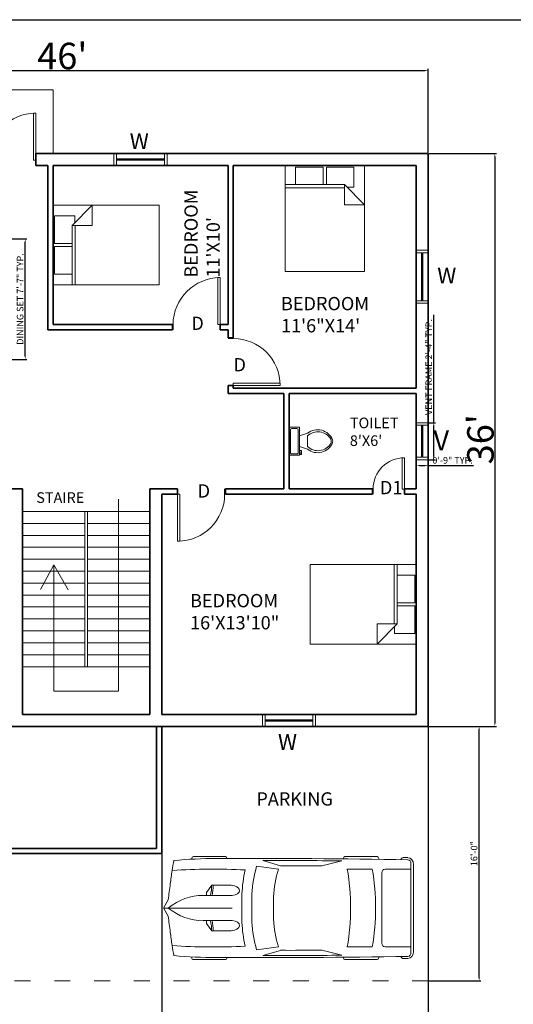
# Model space of a CAD drawing. Units: inches. Extents: x 1662 to 23131, y 1265 to 19127.
# Tile 25 of 26: x 22232 to 22604, y 18361 to 19104. Entities that reach past the tile are written whole.
import ezdxf

# ---------------------------------------------------------------- set-up
doc = ezdxf.new("R2010")
doc.units = ezdxf.units.IN
doc.linetypes.add('ACAD_ISO03W100', pattern=[30, 12, -18])
for name, color, linetype, lineweight in [('A-ANNO-DIMS', 4, 'Continuous', 18), ('A-ANNO-IDEN', 7, 'Continuous', 18), ('A-ANNO-TTLB', 7, 'Continuous', 25), ('A-AREA-IDEN', 7, 'Continuous', 18), ('A-DOOR', 3, 'Continuous', 18), ('A-FLOR-FIXT', 9, 'Continuous', 18), ('A-FLOR-STRS', 7, 'Continuous', 18), ('A-FURN', 8, 'Continuous', 18), ('A-GLAZ', 4, 'Continuous', 18), ('A-SITE-PRKG', 8, 'ACAD_ISO03W100', 18), ('A-SITE-VEHC', 8, 'Continuous', 18), ('A-WALL', 7, 'Continuous', 35)]:
    doc.layers.add(name, color=color, linetype=linetype, lineweight=lineweight)
doc.styles.get("Standard").update_dxf_attribs({"font": 'arial.ttf'})
doc.dimstyles.new('ISO-25', dxfattribs={"dimtxt": 5, "dimasz": 2.5, "dimexe": 1.25, "dimexo": 0.625, "dimtad": 1, "dimlunit": 3, "dimtxsty": 'Standard', "dimcen": 2.5, "dimadec": 0, "dimazin": 0, "dimtfac": 1, "dimtmove": 0, "dimatfit": 3, "dimfxl": 1, "dimarcsym": 0})

# ---------------------------------------------------------------- blocks, each defined once
blk = doc.blocks.new('*U117')
for p, q in [((0, 0), (0, 100)), ((900, 0), (900, 100))]:
    blk.add_line(p, q)
blk.add_lwpolyline([(0, 0), (0, -900), (43.75, -900), (43.75, 0)], close=True)
blk.add_arc((0, 0), 900, 270, 0)
blk = doc.blocks.new('*U121')
for p, q in [((0, 0), (0, -100)), ((-900, 0), (-900, -100))]:
    blk.add_line(p, q)
blk.add_lwpolyline([(0, 0), (0, 900), (-43.75, 900), (-43.75, 0)], close=True)
blk.add_arc((0, 0), 900, 90, 180)
blk = doc.blocks.new('*U120')
for p, q in [((0, 0), (0, -100)), ((-900, 0), (-900, -100))]:
    blk.add_line(p, q)
blk.add_lwpolyline([(0, 0), (0, 900), (-43.75, 900), (-43.75, 0)], close=True)
blk.add_arc((0, 0), 900, 90, 180)
blk = doc.blocks.new('*U118')
for p, q in [((-600, 0), (-600, -100)), ((0, 0), (0, -100))]:
    blk.add_line(p, q)
blk.add_lwpolyline([(0, 0), (0, 600), (-43.75, 600), (-43.75, 0)], close=True)
blk.add_arc((0, 0), 600, 90, 180)
blk = doc.blocks.new('Bed - Queen')
for p, q in [((0, -80.00003), (0, 0)), ((0, 0), (59.99999, 0)), ((59.99999, 0), (59.99999, -80.00003)), ((7.99999, -1.2), (28.79998, -1.2)), ((7.99999, -14.4), (7.99999, -1.2)), ((28.79998, -1.2), (28.79998, -14.4)), ((31.19999, -1.2), (51.99999, -1.2)), ((31.19999, -14.4), (31.19999, -1.2)), ((51.99999, -1.2), (51.99999, -16.4)), ((0, -14.4), (44.8, -14.4)), ((59.99999, -29.6), (44.8, -14.4)), ((44.8, -14.4), (44.8, -29.6)), ((44.8, -16.8), (0, -16.8)), ((51.99999, -16.4), (46.79936, -16.4)), ((44.8, -29.6), (59.99999, -29.6)), ((59.99999, -80.00003), (0, -80.00003))]:
    blk.add_line(p, q)
blk = doc.blocks.new('Toilet - top')
for p, q in [((9.5, -6), (9.5, -2)), ((-10, -8.5), (-8, -8.5)), ((-10, -9.5), (-10, -8.5)), ((-7, -9.5), (-10, -9.5)), ((-8, -8.5), (-8, -8)), ((-7, -8), (-7, -9.5)), ((-4, -8), (-6, -14)), ((4, -14), (-4, -14)), ((4, -8), (6, -14))]:
    blk.add_line(p, q)
blk.add_lwpolyline([(10.5, -8), (10.5, 0), (-10.5, 0), (-10.5, -8)], close=True)
for points in [[(-9.5, -2), (-9.5, -6)], [(8.5, -1), (-8.5, -1)], [(-8.5, -7), (8.5, -7)]]:
    blk.add_lwpolyline(points)
for centre, radius, start, end in [((-8.62, -1.88), 0.884, 81.8699, 188.1301), ((-8.62, -6.12), 0.884, 171.8699, 278.1301), ((8.62, -1.88), 0.884, 351.8699, 98.1301), ((8.62, -6.12), 0.884, 261.8699, 8.1301), ((3.52, -21.58), 12.17, 141.46911, 247.97143), ((4.2, -21.82), 11.33, 136.36773, 238.94682), ((-3.52, -21.58), 12.17, 292.02843, 38.53071), ((-4.2, -21.82), 11.33, 301.05301, 43.63209), ((0, -27.88), 4, 245.73182, 294.26817), ((0, -29), 4, 254.86053, 285.13947)]:
    blk.add_arc(centre, radius, start, end)
blk = doc.blocks.new('*U66')
for p, q in [((536, 950), (536, 936)), ((1182, 988), (568, 988)), ((1214, 950), (1214, 950)), ((3440, 942), (3440, 950)), ((3472, 988), (4087, 988)), ((4119, 950), (4119, 934)), ((1779, 801), (2195, 746)), ((2235, 810), (1899, 912)), ((3412, 904), (3030, 807)), ((4736, -851), (4736, 851)), ((4785, -832), (4785, 832)), ((3516, 746), (3994, 746)), ((4179, 670), (4179, -670)), ((4736, 746), (4242, 746)), ((820, 295), (918, 436)), ((918, 436), (1294, 436)), ((756, 241), (1313, 241)), ((816, 241), (816, 283)), ((1496, -274), (1496, 274)), ((1690, -267), (1690, 267)), ((2102, 216), (2102, -216)), ((4736, -267), (4736, 267)), ((83, 156), (3, 10)), ((0, 0), (1313, 0)), ((3, -10), (83, -156)), ((756, -241), (1313, -241)), ((816, -241), (816, -283)), ((820, -295), (918, -436)), ((918, -436), (1294, -436)), ((2195, -746), (1779, -801)), ((3994, -746), (3516, -746)), ((4242, -746), (4736, -746)), ((536, -950), (536, -936)), ((2235, -810), (1899, -912)), ((3412, -904), (3030, -807)), ((3440, -942), (3440, -950)), ((4119, -950), (4119, -934)), ((1182, -988), (568, -988)), ((1214, -950), (1214, -950)), ((3472, -988), (4087, -988))]:
    blk.add_line(p, q)
for centre, major_axis, ratio, start_param, end_param in [((1046, -12468), (0, 13417), 0.842304, 0.00281, 0.075598), ((568, 950), (0, -37.6), 0.842304, 3.141593, 4.712389), ((1638, -268113), (0, 269063), 0.842304, -0.013397, 0.002797), ((1182, 950), (0, 37.6), 0.842304, -1.570796, 0), ((3472, 950), (0, -37.6), 0.842304, 3.141593, 4.712389), ((4087, 950), (0, 37.6), 0.842304, -1.570796, 0), ((4588, 910), (0, 56.4), 0.842304, -0.013017, 1.249894), ((1638, -268131), (0, 269121), 0.842304, -0.013397, -0.013017), ((4673, 832), (0, -133), 0.842304, 1.570796, 3.128196), ((6757, -699), (0, 7958), 0.842304, 1.367076, 1.39176), ((952, -15087), (0, -15833), 0.842304, 3.096046, 3.200911), ((3436, 137), (0, 2077), 0.842304, 1.245306, 1.50788), ((1638, -268113), (0, -269025), 0.842304, 3.133765, 3.140441), ((2433, -93125), (0, -93935), 0.842304, 3.134049, 3.144098), ((4673, 851), (0, -75.2), 0.842304, 1.570796, 3.128196), ((6583, -699), (0, -7755), 0.842304, 4.528606, 4.561838), ((3414, 137), (0, -2280), 0.842304, 4.449482, 4.652344), ((3800, 71), (0, -2021), 0.842304, 4.372215, 4.640744), ((434, 0), (0, 3734), 0.842304, 4.511394, 4.913384), ((912, 0), (0, 3734), 0.842304, 4.511394, 4.913384), ((4242, 670), (0, 75.2), 0.842304, 0, 1.570796), ((-5194, 1331), (0, -6374), 0.842304, 1.385369, 1.434372), ((331, 432), (0, 696), 0.842304, 4.435146, 4.718221), ((361, 432), (0, 696), 0.842304, 4.435146, 4.718221), ((1290, 339), (161, -9), 0.603834, -1.395552, 1.581315), ((756, -1185), (0, 1427), 0.842304, 0, 0.590319), ((832, 283), (0, 18.8), 0.842304, 0.879714, 1.570796), ((16, 0), (0, -18.8), 0.842304, 4.131459, 5.293319), ((-5194, -1331), (0, 6374), 0.842304, -1.434372, -1.385369), ((756, 1185), (0, 1427), 0.842304, 2.551274, 3.141593), ((832, -283), (0, -18.8), 0.842304, 4.712389, 5.403472), ((331, -432), (0, -696), 0.842304, 1.564964, 1.848039), ((361, -432), (0, -696), 0.842304, 1.564964, 1.848039), ((3414, -137), (0, -2280), 0.842304, -1.510751, -1.307889), ((3436, -137), (0, -2077), 0.842304, -1.50788, -1.245306), ((3800, -71), (0, -2021), 0.842304, -1.499151, -1.230623), ((6583, 699), (0, 7755), 0.842304, 1.721348, 1.754579), ((6757, 699), (0, 7958), 0.842304, 1.749832, 1.774517), ((952, 15087), (0, -15833), 0.842304, -0.059319, 0.045547), ((4242, -670), (0, -75.2), 0.842304, 4.712389, 6.283185), ((1046, 12468), (0, -13417), 0.842304, -0.075598, -0.00281), ((1638, 268113), (0, 269063), 0.842304, 3.138796, 3.15499), ((1638, 268113), (0, -269025), 0.842304, 0.001152, 0.007828), ((2433, 93125), (0, -93935), 0.842304, -0.002505, 0.007544), ((4588, -910), (0, -56.4), 0.842304, -1.249894, 0.013017), ((4673, -851), (0, 75.2), 0.842304, 3.15499, 4.712389), ((4673, -832), (0, -133), 0.842304, 0.013397, 1.570796), ((568, -950), (0, 37.6), 0.842304, 1.570796, 3.141593), ((1182, -950), (0, -37.6), 0.842304, 0, 1.570796), ((3472, -950), (0, -37.6), 0.842304, -1.570796, 0), ((4087, -950), (0, 37.6), 0.842304, 3.141593, 4.712389), ((1638, 268131), (0, 269121), 0.842304, 3.15461, 3.15499)]:
    blk.add_ellipse(centre, major_axis=major_axis, ratio=ratio, start_param=start_param, end_param=end_param)
at = {"extrusion": (0, 0, -1)}
blk.add_ellipse((1290, -339), major_axis=(161, 9), ratio=0.603834, start_param=-1.395552, end_param=1.581315, dxfattribs=at)
blk = doc.blocks.new('*D123')
at = {"layer": 'A-ANNO-DIMS', "color": 0, "lineweight": -2, "transparency": 16777216}
for p, q in [((22540.77, 19002.71), (22591.62, 19002.71)), ((22590.37, 19000.21), (22590.37, 18573.21)), ((22540.77, 18570.71), (22591.62, 18570.71))]:
    blk.add_line(p, q, dxfattribs=at)
at = {"layer": 'A-ANNO-DIMS', "color": 0, "transparency": 16777216}
for points in [[(22589.95, 19000.21), (22590.78, 19000.21), (22590.37, 19002.71)], [(22589.95, 18573.21), (22590.78, 18573.21), (22590.37, 18570.71)]]:
    blk.add_solid(points, dxfattribs=at)
at = {"layer": 'Defpoints', "color": 0, "transparency": 16777216}
for p in [(22540.15, 19002.71), (22540.15, 18570.71), (22590.37, 18570.71)]:
    blk.add_point(p, dxfattribs=at)
at = {"layer": 'A-ANNO-DIMS', "color": 0, "transparency": 16777216, "insert": (22579.52, 18787.23), "char_height": 5, "attachment_point": 5, "rotation": 90}
blk.add_mtext("{\\H4x;36'}", dxfattribs=at)
blk = doc.blocks.new('*D124')
at = {"layer": 'A-ANNO-DIMS', "color": 0, "lineweight": -2, "transparency": 16777216}
for p, q in [((21988.15, 19003.33), (21988.15, 19066.63)), ((21990.65, 19065.38), (22537.65, 19065.38)), ((22540.15, 19003.33), (22540.15, 19066.63))]:
    blk.add_line(p, q, dxfattribs=at)
at = {"layer": 'A-ANNO-DIMS', "color": 0, "transparency": 16777216}
for points in [[(21990.65, 19065.79), (21990.65, 19064.96), (21988.15, 19065.38)], [(22537.65, 19065.79), (22537.65, 19064.96), (22540.15, 19065.38)]]:
    blk.add_solid(points, dxfattribs=at)
at = {"layer": 'Defpoints', "color": 0, "transparency": 16777216}
for p in [(22540.15, 19065.38), (21988.15, 19002.71), (22540.15, 19002.71)]:
    blk.add_point(p, dxfattribs=at)
at = {"layer": 'A-ANNO-DIMS', "color": 0, "transparency": 16777216, "insert": (22264.15, 19076.21), "char_height": 5, "attachment_point": 5}
blk.add_mtext("{\\H4x;46'}", dxfattribs=at)
blk = doc.blocks.new('VENT-24-J9X2')
for p, q in [((9, 28), (0, 28)), ((9, 26), (0, 26)), ((4, 26), (4, 2)), ((4.5, 26), (4.5, 2)), ((5, 26), (5, 2)), ((9, 2), (0, 2)), ((9, 0), (0, 0))]:
    blk.add_line(p, q)
blk = doc.blocks.new('WIN-36-J9X2')
for p, q in [((0, 0), (0, 9)), ((2, 0), (2, 9)), ((38, 0), (38, 9)), ((40, 0), (40, 9)), ((38, 5), (2, 5)), ((38, 4.5), (2, 4.5)), ((38, 4), (2, 4))]:
    blk.add_line(p, q)
blk = doc.blocks.new('*D177')
at = {"layer": 'A-ANNO-DIMS', "color": 0, "lineweight": -2, "transparency": 16777216}
for p, q in [((22223.17, 18938.46), (22237.45, 18938.46)), ((22236.2, 18849.96), (22236.2, 18935.96)), ((22223.17, 18847.46), (22237.45, 18847.46))]:
    blk.add_line(p, q, dxfattribs=at)
at = {"layer": 'A-ANNO-DIMS', "color": 0, "transparency": 16777216}
for points in [[(22235.78, 18935.96), (22236.62, 18935.96), (22236.2, 18938.46)], [(22235.78, 18849.96), (22236.62, 18849.96), (22236.2, 18847.46)]]:
    blk.add_solid(points, dxfattribs=at)
at = {"layer": 'Defpoints', "color": 0, "transparency": 16777216}
for p in [(22222.55, 18938.46), (22236.2, 18938.46), (22222.55, 18847.46)]:
    blk.add_point(p, dxfattribs=at)
at = {"layer": 'A-ANNO-DIMS', "color": 0, "transparency": 16777216, "insert": (22232.99, 18892.96), "char_height": 5, "attachment_point": 5, "rotation": 90}
blk.add_mtext('DINING SET 7\'-7" TYP.', dxfattribs=at)
blk = doc.blocks.new('*D181')
at = {"layer": 'A-ANNO-DIMS', "color": 0, "lineweight": -2, "transparency": 16777216}
for p, q in [((22544.35, 18799.71), (22544.35, 18881.15)), ((22540.77, 18799.71), (22545.6, 18799.71)), ((22544.35, 18774.21), (22544.35, 18797.21)), ((22540.77, 18771.71), (22545.6, 18771.71))]:
    blk.add_line(p, q, dxfattribs=at)
at = {"layer": 'A-ANNO-DIMS', "color": 0, "transparency": 16777216}
for points in [[(22543.93, 18797.21), (22544.77, 18797.21), (22544.35, 18799.71)], [(22543.93, 18774.21), (22544.77, 18774.21), (22544.35, 18771.71)]]:
    blk.add_solid(points, dxfattribs=at)
at = {"layer": 'Defpoints', "color": 0, "transparency": 16777216}
for p in [(22540.15, 18799.71), (22544.35, 18799.71), (22540.15, 18771.71)]:
    blk.add_point(p, dxfattribs=at)
at = {"layer": 'A-ANNO-DIMS', "color": 0, "transparency": 16777216, "insert": (22541.21, 18841.68), "char_height": 5, "attachment_point": 5, "rotation": 90}
blk.add_mtext('VENT FRAME 2\'-4" TYP.', dxfattribs=at)
blk = doc.blocks.new('*D182')
at = {"layer": 'A-ANNO-DIMS', "color": 0, "lineweight": -2, "transparency": 16777216}
for p, q in [((22531.15, 18771.08), (22531.15, 18766.26)), ((22540.15, 18771.08), (22540.15, 18766.26)), ((22533.65, 18767.51), (22537.65, 18767.51)), ((22540.15, 18767.51), (22574.38, 18767.51))]:
    blk.add_line(p, q, dxfattribs=at)
at = {"layer": 'A-ANNO-DIMS', "color": 0, "transparency": 16777216}
for points in [[(22533.65, 18767.93), (22533.65, 18767.09), (22531.15, 18767.51)], [(22537.65, 18767.93), (22537.65, 18767.09), (22540.15, 18767.51)]]:
    blk.add_solid(points, dxfattribs=at)
at = {"layer": 'Defpoints', "color": 0, "transparency": 16777216}
for p in [(22531.15, 18771.71), (22540.15, 18771.71), (22540.15, 18767.51)]:
    blk.add_point(p, dxfattribs=at)
at = {"layer": 'A-ANNO-DIMS', "color": 0, "transparency": 16777216, "insert": (22558.51, 18770.69), "char_height": 5, "attachment_point": 5}
blk.add_mtext('0\'-9" TYP.', dxfattribs=at)
blk = doc.blocks.new('*D255')
at = {"layer": 'A-ANNO-DIMS', "color": 0, "lineweight": -2, "transparency": 16777216}
for p, q in [((22339.15, 18570.08), (22339.15, 18310.24)), ((22540.15, 18570.08), (22540.15, 18310.24)), ((22341.65, 18311.49), (22537.65, 18311.49))]:
    blk.add_line(p, q, dxfattribs=at)
at = {"layer": 'A-ANNO-DIMS', "color": 0, "transparency": 16777216}
for points in [[(22341.65, 18311.91), (22341.65, 18311.08), (22339.15, 18311.49)], [(22537.65, 18311.91), (22537.65, 18311.08), (22540.15, 18311.49)]]:
    blk.add_solid(points, dxfattribs=at)
at = {"layer": 'Defpoints', "color": 0, "transparency": 16777216}
for p in [(22339.15, 18570.71), (22540.15, 18570.71), (22540.15, 18311.49)]:
    blk.add_point(p, dxfattribs=at)
at = {"layer": 'A-ANNO-DIMS', "color": 0, "transparency": 16777216, "insert": (22439.65, 18314.67), "char_height": 5, "attachment_point": 5}
blk.add_mtext('16\'-9"', dxfattribs=at)
blk = doc.blocks.new('*D256')
at = {"layer": 'A-ANNO-DIMS', "color": 0, "lineweight": -2, "transparency": 16777216}
for p, q in [((22540.77, 18570.71), (22579.8, 18570.71)), ((22578.55, 18381.21), (22578.55, 18568.21)), ((22540.77, 18378.71), (22579.8, 18378.71))]:
    blk.add_line(p, q, dxfattribs=at)
at = {"layer": 'A-ANNO-DIMS', "color": 0, "transparency": 16777216}
for points in [[(22578.13, 18568.21), (22578.97, 18568.21), (22578.55, 18570.71)], [(22578.13, 18381.21), (22578.97, 18381.21), (22578.55, 18378.71)]]:
    blk.add_solid(points, dxfattribs=at)
at = {"layer": 'Defpoints', "color": 0, "transparency": 16777216}
for p in [(22540.15, 18570.71), (22578.55, 18570.71), (22540.15, 18378.71)]:
    blk.add_point(p, dxfattribs=at)
at = {"layer": 'A-ANNO-DIMS', "color": 0, "transparency": 16777216, "insert": (22575.37, 18474.71), "char_height": 5, "attachment_point": 5, "rotation": 90}
blk.add_mtext('16\'-0"', dxfattribs=at)

msp = doc.modelspace()

# ---------------------------------------------------------------- linework, layer by layer
at = {"layer": 'A-ANNO-TTLB'}
msp.add_lwpolyline([(21860.989, 19103.605), (23130.86, 19103.605), (23130.86, 17867.351), (21860.989, 17867.351)], close=True, dxfattribs=at)
at = {"layer": 'A-FLOR-STRS'}
for p, q in [((22257.149, 19050.71), (22161.274, 19050.71)), ((22257.149, 19002.71), (22257.149, 19050.71)), ((22306.649, 18742.121), (22306.649, 18597.14)), ((22330.149, 18732.71), (22234.149, 18732.71)), ((22281.149, 18615.71), (22281.149, 18732.71)), ((22283.149, 18615.71), (22283.149, 18732.71)), ((22281.149, 18723.71), (22234.149, 18723.71)), ((22330.149, 18723.71), (22283.149, 18723.71)), ((22281.149, 18714.71), (22234.149, 18714.71)), ((22330.149, 18714.71), (22283.149, 18714.71)), ((22281.149, 18705.71), (22234.149, 18705.71)), ((22330.149, 18705.71), (22283.149, 18705.71)), ((22281.149, 18696.71), (22234.149, 18696.71)), ((22330.149, 18696.71), (22283.149, 18696.71)), ((22257.649, 18692.581), (22247.631, 18673.83)), ((22257.649, 18597.14), (22257.649, 18692.581)), ((22257.649, 18692.581), (22268.486, 18673.708)), ((22281.149, 18687.71), (22234.149, 18687.71)), ((22330.149, 18687.71), (22283.149, 18687.71)), ((22281.149, 18678.71), (22234.149, 18678.71)), ((22330.149, 18678.71), (22283.149, 18678.71)), ((22281.149, 18669.71), (22234.149, 18669.71)), ((22330.149, 18669.71), (22283.149, 18669.71)), ((22281.149, 18660.71), (22234.149, 18660.71)), ((22330.149, 18660.71), (22283.149, 18660.71)), ((22281.149, 18651.71), (22234.149, 18651.71)), ((22330.149, 18651.71), (22283.149, 18651.71)), ((22281.149, 18642.71), (22234.149, 18642.71)), ((22330.149, 18642.71), (22283.149, 18642.71)), ((22281.149, 18633.71), (22234.149, 18633.71)), ((22330.149, 18633.71), (22283.149, 18633.71)), ((22281.149, 18624.71), (22234.149, 18624.71)), ((22330.149, 18624.71), (22283.149, 18624.71)), ((22330.149, 18615.71), (22234.149, 18615.71)), ((22306.649, 18597.14), (22257.649, 18597.14))]:
    msp.add_line(p, q, dxfattribs=at)
at = {"layer": 'A-SITE-PRKG'}
for p, q in [((22540.149, 18570.71), (22540.149, 18378.71)), ((22540.149, 18378.71), (21988.149, 18378.71))]:
    msp.add_line(p, q, dxfattribs=at)
at = {"layer": 'A-WALL'}
for p, q in [((22244.149, 18993.71), (22244.149, 19002.71)), ((22244.149, 19002.71), (22540.149, 19002.71)), ((22540.149, 19002.71), (22540.149, 18570.71)), ((22244.149, 18993.71), (22253.149, 18993.71)), ((22253.149, 18869.71), (22253.149, 18993.71)), ((22257.149, 18873.71), (22257.149, 18993.71)), ((22257.149, 18993.71), (22389.149, 18993.71)), ((22389.149, 18873.71), (22389.149, 18993.71)), ((22393.149, 18863.71), (22393.149, 18993.71)), ((22393.149, 18993.71), (22531.149, 18993.71)), ((22531.149, 18993.71), (22531.149, 18825.71)), ((22253.149, 18869.71), (22347.149, 18869.71)), ((22257.149, 18873.71), (22347.149, 18873.71)), ((22347.149, 18869.71), (22347.149, 18873.71)), ((22383.149, 18869.71), (22383.149, 18873.71)), ((22383.149, 18873.71), (22389.149, 18873.71)), ((22383.149, 18869.71), (22389.149, 18869.71)), ((22389.149, 18863.71), (22389.149, 18869.71)), ((22389.149, 18863.71), (22393.149, 18863.71)), ((22389.149, 18821.71), (22389.149, 18827.71)), ((22389.149, 18827.71), (22393.149, 18827.71)), ((22393.149, 18825.71), (22393.149, 18827.71)), ((22393.149, 18825.71), (22531.149, 18825.71)), ((22389.149, 18821.71), (22431.149, 18821.71)), ((22431.149, 18821.71), (22431.149, 18749.71)), ((22435.149, 18821.71), (22435.149, 18749.71)), ((22435.149, 18821.71), (22531.149, 18821.71)), ((22531.149, 18821.71), (22531.149, 18749.71)), ((22225.149, 18749.71), (22234.149, 18749.71)), ((22234.149, 18579.71), (22234.149, 18749.71)), ((22330.149, 18749.71), (22330.149, 18579.71)), ((22330.149, 18749.71), (22351.149, 18749.71)), ((22351.149, 18749.71), (22351.149, 18745.71)), ((22387.149, 18749.71), (22387.149, 18745.71)), ((22387.149, 18749.71), (22419.149, 18749.71)), ((22419.149, 18749.71), (22431.149, 18749.71)), ((22435.149, 18749.71), (22498.149, 18749.71)), ((22498.149, 18745.71), (22498.149, 18749.71)), ((22522.149, 18745.71), (22522.149, 18749.71)), ((22522.149, 18749.71), (22531.149, 18749.71)), ((22339.149, 18745.71), (22339.149, 18579.71)), ((22339.149, 18745.71), (22351.149, 18745.71)), ((22387.149, 18745.71), (22419.149, 18745.71)), ((22419.149, 18745.71), (22498.149, 18745.71)), ((22522.149, 18745.71), (22531.149, 18745.71)), ((22531.149, 18745.71), (22531.149, 18579.71)), ((22531.149, 18662.71), (22531.149, 18662.71)), ((22330.149, 18579.71), (22234.149, 18579.71)), ((22531.149, 18579.71), (22339.149, 18579.71)), ((22540.149, 18570.71), (22213.149, 18570.71)), ((22335.149, 18570.71), (22335.149, 18478.71)), ((22339.149, 18570.71), (22339.149, 18474.71)), ((22339.149, 18474.71), (22079.649, 18474.71)), ((22335.149, 18478.71), (22083.649, 18478.71))]:
    msp.add_line(p, q, dxfattribs=at)

# ---------------------------------------------------------------- block references
at = {"layer": 'A-DOOR', "xscale": 0.0393700787401575, "yscale": 0.0393700787401575, "zscale": 0.0393700787401575}
for name, p in [('*U121', (22244.149, 18997.647)), ('*U121', (22383.149, 18873.647)), ('*U118', (22522.149, 18749.647)), ('*U117', (22351.149, 18745.773))]:
    msp.add_blockref(name, p, dxfattribs=at)
at = {"layer": 'A-DOOR', "xscale": 0.0393700787401575, "yscale": 0.0393700787401575, "zscale": 0.0393700787401575, "rotation": 270}
msp.add_blockref('*U120', (22393.086, 18827.71), dxfattribs=at)
at = {"layer": 'A-FLOR-FIXT', "rotation": 90}
msp.add_blockref('Toilet - top', (22435.149, 18785.71), dxfattribs=at)
at = {"layer": 'A-FURN'}
msp.add_blockref('Bed - Queen', (22432.149, 18993.71), dxfattribs=at)
for p, rotation in [((22257.149, 18903.71), 89.99999999999999), ((22531.149, 18692.71), 270)]:
    msp.add_blockref('Bed - Queen', p, dxfattribs=dict(at, rotation=rotation))
at = {"layer": 'A-GLAZ'}
for name, p in [('WIN-36-J9X2', (22303.149, 18993.71)), ('VENT-24-J9X2', (22531.149, 18771.71)), ('WIN-36-J9X2', (22415.149, 18570.71))]:
    msp.add_blockref(name, p, dxfattribs=at)
at = {"layer": 'A-GLAZ', "rotation": 90}
msp.add_blockref('WIN-36-J9X2', (22540.149, 18889.709), dxfattribs=at)
at = {"layer": 'A-SITE-VEHC', "xscale": 0.0393700787401575, "yscale": 0.0393700787401575, "zscale": 0.0393700787401575}
msp.add_blockref('*U66', (22340.677, 18433.685), dxfattribs=at)

# ---------------------------------------------------------------- texts
at = {"layer": 'A-ANNO-IDEN', "attachment_point": 1}
for s, width, heights, insert, char_height in [('W', 471.52273, [28.462], (22315.012, 19018.01), 12), ('W', 471.52273, [28.462], (22546.949, 18916.716), 12), ('D', 1142.59551, [0], (22361.493, 18879.666), 10), ('D', 1142.59551, [0], (22393.28, 18848.385), 10), ('V', 1142.59551, [20], (22544.061, 18793.863), 15), ('D', 1142.59551, [0], (22366.243, 18753.244), 10), ('D1', 1142.59551, [20], (22503.712, 18755.755), 10), ('W', 471.52273, [28.462], (22426.818, 18564.969), 12)]:
    msp.add_mtext_dynamic_manual_height_columns(s, width=width, gutter_width=12.5, heights=heights, dxfattribs=dict(at, insert=insert, char_height=char_height))
at = {"layer": 'A-AREA-IDEN', "insert": (22356.264, 18909.08), "char_height": 10, "attachment_point": 1, "rotation": 90}
msp.add_mtext_dynamic_manual_height_columns("BEDROOM\\P11'X10'", width=1142.59551, gutter_width=12.5, heights=[277.772], dxfattribs=at)
at = {"layer": 'A-AREA-IDEN', "attachment_point": 1}
for s, insert, char_height in [('BEDROOM\\P11\'6"X14\'', (22429.103, 18894.49), 10), ("TOILET\\P8'X6'", (22481.026, 18803.516), 8), ('STAIRE', (22244.504, 18747.208), 8), ('BEDROOM\\P16\'X13\'10"', (22360.517, 18670.489), 10), ('PARKING', (22410.538, 18520.968), 10)]:
    msp.add_mtext_dynamic_manual_height_columns(s, width=1142.59551, gutter_width=12.5, heights=[277.772], dxfattribs=dict(at, insert=insert, char_height=char_height))

# ---------------------------------------------------------------- dimensions: what is measured, and where the dimension line sits
at = {"layer": 'A-ANNO-DIMS'}
for base, p1, p2, text, override, picture, middle in [((22540.149, 19065.376), (21988.149, 19002.71), (22540.149, 19002.71), '{\\H4x;<>}', {"dimclrd": 0, "dimclre": 0, "dimclrt": 0}, '*D124', (22264.149, 19076.213)), ((22540.149, 18767.51), (22531.149, 18771.71), (22540.149, 18771.71), '<> TYP.', {"dimdec": 1, "dimlfac": 1, "dimrnd": 0, "dimzin": 1, "dimdsep": 46, "dimlunit": 4, "dimfrac": 2}, '*D182', (22558.513, 18770.687))]:
    dim = msp.add_linear_dim(base=base, p1=p1, p2=p2, text=text, dimstyle='ISO-25', override=override, dxfattribs=at)
    dim.commit()
    dim.dimension.update_dxf_attribs({"geometry": picture, "text_midpoint": middle})
dim = msp.add_linear_dim(base=(22590.366, 18570.71), p1=(22540.149, 19002.71), p2=(22540.149, 18570.71), angle=90, text='{\\H4x;<>}', dimstyle='ISO-25', override={"dimclrd": 0, "dimclre": 0, "dimclrt": 0}, dxfattribs=at)
dim.commit()
dim.dimension.update_dxf_attribs({"geometry": '*D123', "text_midpoint": (22590.366, 18787.231), "dimtype": 160})
for base, p1, p2, text, picture, middle in [((22236.199, 18938.455), (22222.549, 18847.455), (22222.549, 18938.455), 'DINING SET <> TYP.', '*D177', (22232.989, 18892.955)), ((22544.349, 18799.71), (22540.149, 18771.71), (22540.149, 18799.71), 'VENT FRAME <> TYP.', '*D181', (22541.212, 18841.682))]:
    dim = msp.add_linear_dim(base=base, p1=p1, p2=p2, angle=90, text=text, dimstyle='ISO-25', override={"dimdec": 1, "dimlfac": 1, "dimrnd": 0, "dimzin": 1, "dimdsep": 46, "dimlunit": 4, "dimfrac": 2}, dxfattribs=at)
    dim.commit()
    dim.dimension.update_dxf_attribs({"geometry": picture, "text_midpoint": middle})
dim = msp.add_linear_dim(base=(22540.149, 18311.495), p1=(22339.149, 18570.71), p2=(22540.149, 18570.71), dimstyle='ISO-25', override={"dimdec": 1, "dimlfac": 1, "dimrnd": 0, "dimzin": 1, "dimdsep": 46, "dimlunit": 4, "dimfrac": 2}, dxfattribs=at)
dim.commit()
dim.dimension.update_dxf_attribs({"geometry": '*D255', "text_midpoint": (22439.649, 18314.673)})
dim = msp.add_linear_dim(base=(22578.549, 18570.71), p1=(22540.149, 18378.71), p2=(22540.149, 18570.71), angle=90, dimstyle='ISO-25', override={"dimdec": 1, "dimlfac": 1, "dimrnd": 0, "dimzin": 1, "dimdsep": 46, "dimlunit": 4, "dimfrac": 2}, dxfattribs=at)
dim.commit()
dim.dimension.update_dxf_attribs({"geometry": '*D256', "text_midpoint": (22575.371, 18474.71)})

doc.saveas('drawing.dxf')
